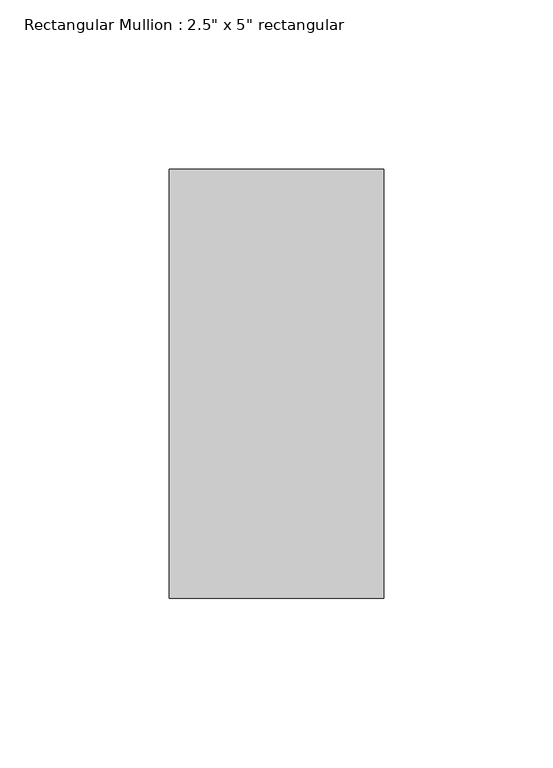
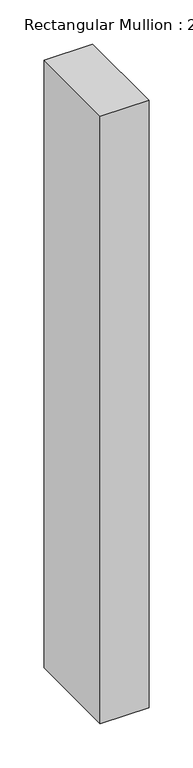
"""IFC4 building model written with IfcOpenShell, lengths in millimetres: member geometry."""

from ifc_helpers import new_model, si_unit, frame, origin, place, context, project, spatial, polyline, outline, extrude, source, transform, mapped, element, save


def member_262c5f3f(model_context):
    return source(origin(), model_context, "Body", "SweptSolid", [
        extrude(outline(polyline([(0.0, 63.5), (0.0, -63.5), (-63.5, -63.5), (-63.5, 63.5), (0.0, 63.5)])), frame((0.0, 0.0, -837.8574877), z_axis=(0.0, 0.0, 1.0), x_axis=(1.0, 0.0, 0.0)), (0.0, 0.0, 1.0), 837.8574877),
    ])


if __name__ == "__main__":
    model = new_model("IFC4")
    model_context = context("Model", 3, world=origin())
    ifc_project = project(units=[si_unit("LENGTHUNIT", "METRE", prefix="MILLI")], contexts=[model_context])
    site = spatial("IfcSite", under=ifc_project)
    building = spatial("IfcBuilding", under=site)
    placement = place(None, origin())
    member_shape = member_262c5f3f(model_context)
    element("IfcMember", 1, ObjectType="Rectangular Mullion : 2.5\" x 5\" rectangular", at=placement, inside=building, context=model_context, shape_type="MappedRepresentation", body=[
        mapped(member_shape, transform((0.0, 0.0, 0.0), x_axis=(1.0, 0.0, 0.0), y_axis=(0.0, 1.0, 0.0), z_axis=(0.0, 0.0, 1.0))),
    ])
    save(model, "model.ifc")

# Revit data of these elements
# Type "Rectangular Mullion : 2.5\" x 5\" rectangular"
#   built-in parameter 1007304 = 0.416667 (stored number, unit not read)
#   built-in parameter 1007301 = 0.104167 (stored number, unit not read)
#   built-in parameter 1007300 = 0.104167 (stored number, unit not read)
# Element 1 (IfcMember, "Rectangular Mullion : 2.5\" x 5\" rectangular")
#   Materials on its faces: "Aluminum"
# Materials
#   "Aluminum": class "Metal", colour RGB 247 247 247, transparency 0, Description = "Aluminum 6061", Cost = 0
